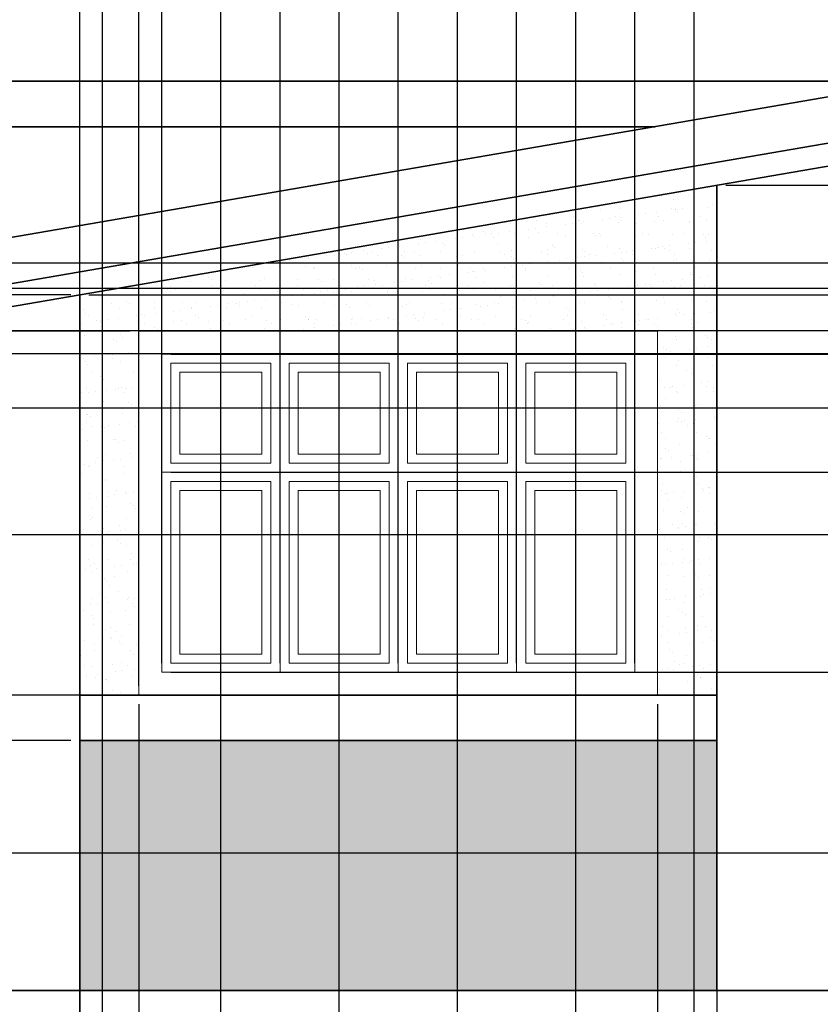
# Model space of a CAD drawing. Units: millimetres. Extents: x 937 to 4561, y 2711 to 5748.
# Tile 3 of 8: x 1663 to 2543, y 4062 to 5145. Entities that reach past the tile are written whole.
import ezdxf

# ---------------------------------------------------------------- set-up
doc = ezdxf.new("R2010")
doc.units = ezdxf.units.MM
doc.header["$MEASUREMENT"] = 0
for name, color, linetype, lineweight in [('A-ANNO-DIMS', 2, 'Continuous', 18), ('A-ELEV', 7, 'Continuous', 35), ('A-GLAZ', 4, 'Continuous', 18), ('A-ROOF', 1, 'Continuous', 35), ('A-WALL-PATT', 8, 'Continuous', 13)]:
    doc.layers.add(name, color=color, linetype=linetype, lineweight=lineweight)
doc.styles.get("Standard").update_dxf_attribs({"font": 'arial.ttf'})
doc.dimstyles.get("Standard").update_dxf_attribs({"dimtxt": 15, "dimasz": 10, "dimexe": 10, "dimexo": 10, "dimgap": 10, "dimtad": 0, "dimtih": 1, "dimtoh": 1, "dimdec": 0, "dimzin": 0, "dimdsep": 46, "dimtxsty": 'Standard', "dimcen": 5, "dimadec": 0, "dimazin": 0, "dimtfac": 1, "dimtdec": 0, "dimtofl": 0, "dimtmove": 0, "dimatfit": 3, "dimfxl": 1, "dimtolj": 1, "dimtzin": 0, "dimarcsym": 0})

# ---------------------------------------------------------------- blocks, each defined once
blk = doc.blocks.new('*D15')
at = {"layer": 'A-ANNO-DIMS', "color": 0, "lineweight": -2, "transparency": 16777216}
for p, q in [((1329.5, 4086.9), (1329.5, 5747.9)), ((4179.5, 5586.9), (4179.5, 5747.9)), ((1339.5, 5737.9), (2722, 5737.9)), ((4169.5, 5737.9), (2787, 5737.9))]:
    blk.add_line(p, q, dxfattribs=at)
at = {"layer": 'A-ANNO-DIMS', "color": 0, "transparency": 16777216}
for points in [[(1339.5, 5739.6), (1339.5, 5736.2), (1329.5, 5737.9)], [(4169.5, 5739.6), (4169.5, 5736.2), (4179.5, 5737.9)]]:
    blk.add_solid(points, dxfattribs=at)
at = {"layer": 'Defpoints', "color": 0, "transparency": 16777216}
for p in [(4179.5, 5737.9), (4179.5, 5576.9), (1329.5, 4076.9)]:
    blk.add_point(p, dxfattribs=at)
at = {"layer": 'A-ANNO-DIMS', "color": 0, "transparency": 16777216, "insert": (2754.5, 5737.9), "char_height": 15, "attachment_point": 5}
blk.add_mtext('\\A1;2850', dxfattribs=at)
blk = doc.blocks.new('*D16')
at = {"layer": 'A-ANNO-DIMS', "color": 0, "lineweight": -2, "transparency": 16777216}
for p, q in [((1329.5, 4859.2), (1329.5, 5747.9)), ((2947.4, 5137.7), (2947.4, 5747.9)), ((1339.5, 5737.9), (2106.8, 5737.9)), ((2937.4, 5737.9), (2170.2, 5737.9))]:
    blk.add_line(p, q, dxfattribs=at)
at = {"layer": 'A-ANNO-DIMS', "color": 0, "transparency": 16777216}
for points in [[(1339.5, 5739.6), (1339.5, 5736.2), (1329.5, 5737.9)], [(2937.4, 5739.6), (2937.4, 5736.2), (2947.4, 5737.9)]]:
    blk.add_solid(points, dxfattribs=at)
at = {"layer": 'Defpoints', "color": 0, "transparency": 16777216}
for p in [(2947.4, 5737.9), (2947.4, 5127.7), (1329.5, 4849.2)]:
    blk.add_point(p, dxfattribs=at)
at = {"layer": 'A-ANNO-DIMS', "color": 0, "transparency": 16777216, "insert": (2138.5, 5737.9), "char_height": 15, "attachment_point": 5}
blk.add_mtext('\\A1;1618', dxfattribs=at)
blk = doc.blocks.new('*D27')
at = {"layer": 'A-ANNO-DIMS', "color": 0, "lineweight": -2, "transparency": 16777216}
for p, q in [((1729.5, 4391.9), (1729.5, 2710.9)), ((1794.5, 4391.9), (1794.5, 2710.9)), ((1719.5, 2720.9), (1709.5, 2720.9)), ((1804.5, 2720.9), (1814.5, 2720.9))]:
    blk.add_line(p, q, dxfattribs=at)
at = {"layer": 'A-ANNO-DIMS', "color": 0, "transparency": 16777216}
for points in [[(1719.5, 2722.6), (1719.5, 2719.2), (1729.5, 2720.9)], [(1804.5, 2722.6), (1804.5, 2719.2), (1794.5, 2720.9)]]:
    blk.add_solid(points, dxfattribs=at)
at = {"layer": 'Defpoints', "color": 0, "transparency": 16777216}
for p in [(1729.5, 4401.9), (1794.5, 4401.9), (1794.5, 2720.9)]:
    blk.add_point(p, dxfattribs=at)
at = {"layer": 'A-ANNO-DIMS', "color": 0, "transparency": 16777216, "insert": (1762, 2720.9), "char_height": 15, "attachment_point": 5}
blk.add_mtext('\\A1;65', dxfattribs=at)
blk = doc.blocks.new('*D28')
at = {"layer": 'A-ANNO-DIMS', "color": 0, "lineweight": -2, "transparency": 16777216}
for p, q in [((1794.5, 4391.9), (1794.5, 2710.9)), ((2364.5, 4391.9), (2364.5, 2710.9)), ((1804.5, 2720.9), (2052.9, 2720.9)), ((2354.5, 2720.9), (2106, 2720.9))]:
    blk.add_line(p, q, dxfattribs=at)
at = {"layer": 'A-ANNO-DIMS', "color": 0, "transparency": 16777216}
for points in [[(1804.5, 2722.6), (1804.5, 2719.2), (1794.5, 2720.9)], [(2354.5, 2722.6), (2354.5, 2719.2), (2364.5, 2720.9)]]:
    blk.add_solid(points, dxfattribs=at)
at = {"layer": 'Defpoints', "color": 0, "transparency": 16777216}
for p in [(1794.5, 4401.9), (2364.5, 4401.9), (2364.5, 2720.9)]:
    blk.add_point(p, dxfattribs=at)
at = {"layer": 'A-ANNO-DIMS', "color": 0, "transparency": 16777216, "insert": (2079.5, 2720.9), "char_height": 15, "attachment_point": 5}
blk.add_mtext('\\A1;570', dxfattribs=at)
blk = doc.blocks.new('*D29')
at = {"layer": 'A-ANNO-DIMS', "color": 0, "lineweight": -2, "transparency": 16777216}
for p, q in [((2364.5, 4391.9), (2364.5, 2710.9)), ((2429.5, 4391.9), (2429.5, 2710.9)), ((2354.5, 2720.9), (2344.5, 2720.9)), ((2439.5, 2720.9), (2449.5, 2720.9))]:
    blk.add_line(p, q, dxfattribs=at)
at = {"layer": 'A-ANNO-DIMS', "color": 0, "transparency": 16777216}
for points in [[(2354.5, 2722.6), (2354.5, 2719.2), (2364.5, 2720.9)], [(2439.5, 2722.6), (2439.5, 2719.2), (2429.5, 2720.9)]]:
    blk.add_solid(points, dxfattribs=at)
at = {"layer": 'Defpoints', "color": 0, "transparency": 16777216}
for p in [(2364.5, 4401.9), (2429.5, 4401.9), (2429.5, 2720.9)]:
    blk.add_point(p, dxfattribs=at)
at = {"layer": 'A-ANNO-DIMS', "color": 0, "transparency": 16777216, "insert": (2397, 2720.9), "char_height": 15, "attachment_point": 5}
blk.add_mtext('\\A1;65', dxfattribs=at)
blk = doc.blocks.new('*D30')
at = {"layer": 'A-ANNO-DIMS', "color": 0, "lineweight": -2, "transparency": 16777216}
for p, q in [((1794.5, 4411.9), (1794.5, 5747.9)), ((1819.5, 4436.9), (1819.5, 5747.9)), ((1784.5, 5737.9), (1774.5, 5737.9)), ((1829.5, 5737.9), (1839.5, 5737.9))]:
    blk.add_line(p, q, dxfattribs=at)
at = {"layer": 'A-ANNO-DIMS', "color": 0, "transparency": 16777216}
for points in [[(1784.5, 5739.6), (1784.5, 5736.2), (1794.5, 5737.9)], [(1829.5, 5739.6), (1829.5, 5736.2), (1819.5, 5737.9)]]:
    blk.add_solid(points, dxfattribs=at)
at = {"layer": 'Defpoints', "color": 0, "transparency": 16777216}
for p in [(1819.5, 5737.9), (1819.5, 4426.9), (1794.5, 4401.9)]:
    blk.add_point(p, dxfattribs=at)
at = {"layer": 'A-ANNO-DIMS', "color": 0, "transparency": 16777216, "insert": (1860.4, 5737.9), "char_height": 15, "attachment_point": 5}
blk.add_mtext('\\A1;25', dxfattribs=at)
blk = doc.blocks.new('*D31')
at = {"layer": 'A-ANNO-DIMS', "color": 0, "lineweight": -2, "transparency": 16777216}
for p, q in [((1819.5, 4436.9), (1819.5, 5747.9)), ((1949.5, 4436.9), (1949.5, 5747.9)), ((1829.5, 5737.9), (1858.6, 5737.9)), ((1939.5, 5737.9), (1910.3, 5737.9))]:
    blk.add_line(p, q, dxfattribs=at)
at = {"layer": 'A-ANNO-DIMS', "color": 0, "transparency": 16777216}
for points in [[(1829.5, 5739.6), (1829.5, 5736.2), (1819.5, 5737.9)], [(1939.5, 5739.6), (1939.5, 5736.2), (1949.5, 5737.9)]]:
    blk.add_solid(points, dxfattribs=at)
at = {"layer": 'Defpoints', "color": 0, "transparency": 16777216}
for p in [(1949.5, 5737.9), (1819.5, 4426.9), (1949.5, 4426.9)]:
    blk.add_point(p, dxfattribs=at)
at = {"layer": 'A-ANNO-DIMS', "color": 0, "transparency": 16777216, "insert": (1884.5, 5737.9), "char_height": 15, "attachment_point": 5}
blk.add_mtext('\\A1;130', dxfattribs=at)
blk = doc.blocks.new('*D32')
at = {"layer": 'A-ANNO-DIMS', "color": 0, "lineweight": -2, "transparency": 16777216}
for p, q in [((1949.5, 4436.9), (1949.5, 5747.9)), ((2079.5, 4436.9), (2079.5, 5747.9)), ((1959.5, 5737.9), (1988.6, 5737.9)), ((2069.5, 5737.9), (2040.3, 5737.9))]:
    blk.add_line(p, q, dxfattribs=at)
at = {"layer": 'A-ANNO-DIMS', "color": 0, "transparency": 16777216}
for points in [[(1959.5, 5739.6), (1959.5, 5736.2), (1949.5, 5737.9)], [(2069.5, 5739.6), (2069.5, 5736.2), (2079.5, 5737.9)]]:
    blk.add_solid(points, dxfattribs=at)
at = {"layer": 'Defpoints', "color": 0, "transparency": 16777216}
for p in [(2079.5, 5737.9), (1949.5, 4426.9), (2079.5, 4426.9)]:
    blk.add_point(p, dxfattribs=at)
at = {"layer": 'A-ANNO-DIMS', "color": 0, "transparency": 16777216, "insert": (2014.5, 5737.9), "char_height": 15, "attachment_point": 5}
blk.add_mtext('\\A1;130', dxfattribs=at)
blk = doc.blocks.new('*D33')
at = {"layer": 'A-ANNO-DIMS', "color": 0, "lineweight": -2, "transparency": 16777216}
for p, q in [((2079.5, 4436.9), (2079.5, 5747.9)), ((2209.5, 4436.9), (2209.5, 5747.9)), ((2089.5, 5737.9), (2118.6, 5737.9)), ((2199.5, 5737.9), (2170.3, 5737.9))]:
    blk.add_line(p, q, dxfattribs=at)
at = {"layer": 'A-ANNO-DIMS', "color": 0, "transparency": 16777216}
for points in [[(2089.5, 5739.6), (2089.5, 5736.2), (2079.5, 5737.9)], [(2199.5, 5739.6), (2199.5, 5736.2), (2209.5, 5737.9)]]:
    blk.add_solid(points, dxfattribs=at)
at = {"layer": 'Defpoints', "color": 0, "transparency": 16777216}
for p in [(2209.5, 5737.9), (2079.5, 4426.9), (2209.5, 4426.9)]:
    blk.add_point(p, dxfattribs=at)
at = {"layer": 'A-ANNO-DIMS', "color": 0, "transparency": 16777216, "insert": (2144.5, 5737.9), "char_height": 15, "attachment_point": 5}
blk.add_mtext('\\A1;130', dxfattribs=at)
blk = doc.blocks.new('*D34')
at = {"layer": 'A-ANNO-DIMS', "color": 0, "lineweight": -2, "transparency": 16777216}
for p, q in [((2209.5, 4436.9), (2209.5, 5747.9)), ((2339.5, 4436.9), (2339.5, 5747.9)), ((2219.5, 5737.9), (2248.6, 5737.9)), ((2329.5, 5737.9), (2300.3, 5737.9))]:
    blk.add_line(p, q, dxfattribs=at)
at = {"layer": 'A-ANNO-DIMS', "color": 0, "transparency": 16777216}
for points in [[(2219.5, 5739.6), (2219.5, 5736.2), (2209.5, 5737.9)], [(2329.5, 5739.6), (2329.5, 5736.2), (2339.5, 5737.9)]]:
    blk.add_solid(points, dxfattribs=at)
at = {"layer": 'Defpoints', "color": 0, "transparency": 16777216}
for p in [(2339.5, 5737.9), (2209.5, 4426.9), (2339.5, 4426.9)]:
    blk.add_point(p, dxfattribs=at)
at = {"layer": 'A-ANNO-DIMS', "color": 0, "transparency": 16777216, "insert": (2274.5, 5737.9), "char_height": 15, "attachment_point": 5}
blk.add_mtext('\\A1;130', dxfattribs=at)
blk = doc.blocks.new('*D37')
at = {"layer": 'A-ANNO-DIMS', "color": 0, "lineweight": -2, "transparency": 16777216}
for p, q in [((1729.5, 3411.9), (1729.5, 5747.9)), ((1754.5, 3436.9), (1754.5, 5747.9)), ((1719.5, 5737.9), (1709.5, 5737.9)), ((1764.5, 5737.9), (1774.5, 5737.9))]:
    blk.add_line(p, q, dxfattribs=at)
at = {"layer": 'A-ANNO-DIMS', "color": 0, "transparency": 16777216}
for points in [[(1719.5, 5739.6), (1719.5, 5736.2), (1729.5, 5737.9)], [(1764.5, 5739.6), (1764.5, 5736.2), (1754.5, 5737.9)]]:
    blk.add_solid(points, dxfattribs=at)
at = {"layer": 'Defpoints', "color": 0, "transparency": 16777216}
for p in [(1754.5, 5737.9), (1754.5, 3426.9), (1729.5, 3401.9)]:
    blk.add_point(p, dxfattribs=at)
at = {"layer": 'A-ANNO-DIMS', "color": 0, "transparency": 16777216, "insert": (1795.4, 5737.9), "char_height": 15, "attachment_point": 5}
blk.add_mtext('\\A1;25', dxfattribs=at)
blk = doc.blocks.new('*D38')
at = {"layer": 'A-ANNO-DIMS', "color": 0, "lineweight": -2, "transparency": 16777216}
for p, q in [((1754.5, 3436.9), (1754.5, 5747.9)), ((1884.5, 3436.9), (1884.5, 5747.9)), ((1764.5, 5737.9), (1793.6, 5737.9)), ((1874.5, 5737.9), (1845.3, 5737.9))]:
    blk.add_line(p, q, dxfattribs=at)
at = {"layer": 'A-ANNO-DIMS', "color": 0, "transparency": 16777216}
for points in [[(1764.5, 5739.6), (1764.5, 5736.2), (1754.5, 5737.9)], [(1874.5, 5739.6), (1874.5, 5736.2), (1884.5, 5737.9)]]:
    blk.add_solid(points, dxfattribs=at)
at = {"layer": 'Defpoints', "color": 0, "transparency": 16777216}
for p in [(1884.5, 5737.9), (1754.5, 3426.9), (1884.5, 3426.9)]:
    blk.add_point(p, dxfattribs=at)
at = {"layer": 'A-ANNO-DIMS', "color": 0, "transparency": 16777216, "insert": (1819.5, 5737.9), "char_height": 15, "attachment_point": 5}
blk.add_mtext('\\A1;130', dxfattribs=at)
blk = doc.blocks.new('*D39')
at = {"layer": 'A-ANNO-DIMS', "color": 0, "lineweight": -2, "transparency": 16777216}
for p, q in [((1884.5, 3436.9), (1884.5, 5747.9)), ((2014.5, 3436.9), (2014.5, 5747.9)), ((1894.5, 5737.9), (1923.6, 5737.9)), ((2004.5, 5737.9), (1975.3, 5737.9))]:
    blk.add_line(p, q, dxfattribs=at)
at = {"layer": 'A-ANNO-DIMS', "color": 0, "transparency": 16777216}
for points in [[(1894.5, 5739.6), (1894.5, 5736.2), (1884.5, 5737.9)], [(2004.5, 5739.6), (2004.5, 5736.2), (2014.5, 5737.9)]]:
    blk.add_solid(points, dxfattribs=at)
at = {"layer": 'Defpoints', "color": 0, "transparency": 16777216}
for p in [(2014.5, 5737.9), (1884.5, 3426.9), (2014.5, 3426.9)]:
    blk.add_point(p, dxfattribs=at)
at = {"layer": 'A-ANNO-DIMS', "color": 0, "transparency": 16777216, "insert": (1949.5, 5737.9), "char_height": 15, "attachment_point": 5}
blk.add_mtext('\\A1;130', dxfattribs=at)
blk = doc.blocks.new('*D40')
at = {"layer": 'A-ANNO-DIMS', "color": 0, "lineweight": -2, "transparency": 16777216}
for p, q in [((2014.5, 3436.9), (2014.5, 5747.9)), ((2144.5, 3436.9), (2144.5, 5747.9)), ((2024.5, 5737.9), (2053.6, 5737.9)), ((2134.5, 5737.9), (2105.3, 5737.9))]:
    blk.add_line(p, q, dxfattribs=at)
at = {"layer": 'A-ANNO-DIMS', "color": 0, "transparency": 16777216}
for points in [[(2024.5, 5739.6), (2024.5, 5736.2), (2014.5, 5737.9)], [(2134.5, 5739.6), (2134.5, 5736.2), (2144.5, 5737.9)]]:
    blk.add_solid(points, dxfattribs=at)
at = {"layer": 'Defpoints', "color": 0, "transparency": 16777216}
for p in [(2144.5, 5737.9), (2014.5, 3426.9), (2144.5, 3426.9)]:
    blk.add_point(p, dxfattribs=at)
at = {"layer": 'A-ANNO-DIMS', "color": 0, "transparency": 16777216, "insert": (2079.5, 5737.9), "char_height": 15, "attachment_point": 5}
blk.add_mtext('\\A1;130', dxfattribs=at)
blk = doc.blocks.new('*D41')
at = {"layer": 'A-ANNO-DIMS', "color": 0, "lineweight": -2, "transparency": 16777216}
for p, q in [((2144.5, 3436.9), (2144.5, 5747.9)), ((2274.5, 3436.9), (2274.5, 5747.9)), ((2154.5, 5737.9), (2183.6, 5737.9)), ((2264.5, 5737.9), (2235.3, 5737.9))]:
    blk.add_line(p, q, dxfattribs=at)
at = {"layer": 'A-ANNO-DIMS', "color": 0, "transparency": 16777216}
for points in [[(2154.5, 5739.6), (2154.5, 5736.2), (2144.5, 5737.9)], [(2264.5, 5739.6), (2264.5, 5736.2), (2274.5, 5737.9)]]:
    blk.add_solid(points, dxfattribs=at)
at = {"layer": 'Defpoints', "color": 0, "transparency": 16777216}
for p in [(2274.5, 5737.9), (2144.5, 3426.9), (2274.5, 3426.9)]:
    blk.add_point(p, dxfattribs=at)
at = {"layer": 'A-ANNO-DIMS', "color": 0, "transparency": 16777216, "insert": (2209.5, 5737.9), "char_height": 15, "attachment_point": 5}
blk.add_mtext('\\A1;130', dxfattribs=at)
blk = doc.blocks.new('*D42')
at = {"layer": 'A-ANNO-DIMS', "color": 0, "lineweight": -2, "transparency": 16777216}
for p, q in [((2274.5, 3436.9), (2274.5, 5747.9)), ((2404.5, 3436.9), (2404.5, 5747.9)), ((2284.5, 5737.9), (2313.6, 5737.9)), ((2394.5, 5737.9), (2365.3, 5737.9))]:
    blk.add_line(p, q, dxfattribs=at)
at = {"layer": 'A-ANNO-DIMS', "color": 0, "transparency": 16777216}
for points in [[(2284.5, 5739.6), (2284.5, 5736.2), (2274.5, 5737.9)], [(2394.5, 5739.6), (2394.5, 5736.2), (2404.5, 5737.9)]]:
    blk.add_solid(points, dxfattribs=at)
at = {"layer": 'Defpoints', "color": 0, "transparency": 16777216}
for p in [(2404.5, 5737.9), (2274.5, 3426.9), (2404.5, 3426.9)]:
    blk.add_point(p, dxfattribs=at)
at = {"layer": 'A-ANNO-DIMS', "color": 0, "transparency": 16777216, "insert": (2339.5, 5737.9), "char_height": 15, "attachment_point": 5}
blk.add_mtext('\\A1;130', dxfattribs=at)
blk = doc.blocks.new('*D43')
at = {"layer": 'A-ANNO-DIMS', "color": 0, "lineweight": -2, "transparency": 16777216}
for p, q in [((1329.5, 4086.9), (1329.5, 5747.9)), ((2579.5, 4086.9), (2579.5, 5747.9)), ((1339.5, 5737.9), (1922.8, 5737.9)), ((2569.5, 5737.9), (1986.2, 5737.9))]:
    blk.add_line(p, q, dxfattribs=at)
at = {"layer": 'A-ANNO-DIMS', "color": 0, "transparency": 16777216}
for points in [[(1339.5, 5739.6), (1339.5, 5736.2), (1329.5, 5737.9)], [(2569.5, 5739.6), (2569.5, 5736.2), (2579.5, 5737.9)]]:
    blk.add_solid(points, dxfattribs=at)
at = {"layer": 'Defpoints', "color": 0, "transparency": 16777216}
for p in [(2579.5, 5737.9), (1329.5, 4076.9), (2579.5, 4076.9)]:
    blk.add_point(p, dxfattribs=at)
at = {"layer": 'A-ANNO-DIMS', "color": 0, "transparency": 16777216, "insert": (1954.5, 5737.9), "char_height": 15, "attachment_point": 5}
blk.add_mtext('\\A1;1250', dxfattribs=at)
blk = doc.blocks.new('*D60')
at = {"layer": 'A-ANNO-DIMS', "color": 0, "lineweight": -2, "transparency": 16777216}
for p, q in [((1784.5, 4401.9), (958.5, 4401.9)), ((968.5, 4391.9), (968.5, 4257.1)), ((968.5, 4086.9), (968.5, 4221.7)), ((1419.5, 4076.9), (958.5, 4076.9))]:
    blk.add_line(p, q, dxfattribs=at)
at = {"layer": 'A-ANNO-DIMS', "color": 0, "transparency": 16777216}
for points in [[(966.8, 4391.9), (970.2, 4391.9), (968.5, 4401.9)], [(966.8, 4086.9), (970.2, 4086.9), (968.5, 4076.9)]]:
    blk.add_solid(points, dxfattribs=at)
at = {"layer": 'Defpoints', "color": 0, "transparency": 16777216}
for p in [(968.5, 4401.9), (1794.5, 4401.9), (1429.5, 4076.9)]:
    blk.add_point(p, dxfattribs=at)
at = {"layer": 'A-ANNO-DIMS', "color": 0, "transparency": 16777216, "insert": (968.5, 4239.4), "char_height": 15, "attachment_point": 5}
blk.add_mtext('\\A1;325', dxfattribs=at)
blk = doc.blocks.new('*D61')
at = {"layer": 'A-ANNO-DIMS', "color": 0, "lineweight": -2, "transparency": 16777216}
for p, q in [((1784.5, 4801.9), (958.5, 4801.9)), ((968.5, 4791.9), (968.5, 4619.6)), ((968.5, 4411.9), (968.5, 4584.2)), ((1784.5, 4401.9), (958.5, 4401.9))]:
    blk.add_line(p, q, dxfattribs=at)
at = {"layer": 'A-ANNO-DIMS', "color": 0, "transparency": 16777216}
for points in [[(966.8, 4791.9), (970.2, 4791.9), (968.5, 4801.9)], [(966.8, 4411.9), (970.2, 4411.9), (968.5, 4401.9)]]:
    blk.add_solid(points, dxfattribs=at)
at = {"layer": 'Defpoints', "color": 0, "transparency": 16777216}
for p in [(968.5, 4801.9), (1794.5, 4801.9), (1794.5, 4401.9)]:
    blk.add_point(p, dxfattribs=at)
at = {"layer": 'A-ANNO-DIMS', "color": 0, "transparency": 16777216, "insert": (968.5, 4601.9), "char_height": 15, "attachment_point": 5}
blk.add_mtext('\\A1;400', dxfattribs=at)
blk = doc.blocks.new('*D62')
at = {"layer": 'A-ANNO-DIMS', "color": 0, "lineweight": -2, "transparency": 16777216}
for p, q in [((1419.5, 5076.9), (958.5, 5076.9)), ((968.5, 5066.9), (968.5, 4957.1)), ((968.5, 4811.9), (968.5, 4921.7)), ((1784.5, 4801.9), (958.5, 4801.9))]:
    blk.add_line(p, q, dxfattribs=at)
at = {"layer": 'A-ANNO-DIMS', "color": 0, "transparency": 16777216}
for points in [[(966.8, 5066.9), (970.2, 5066.9), (968.5, 5076.9)], [(966.8, 4811.9), (970.2, 4811.9), (968.5, 4801.9)]]:
    blk.add_solid(points, dxfattribs=at)
at = {"layer": 'Defpoints', "color": 0, "transparency": 16777216}
for p in [(968.5, 5076.9), (1429.5, 5076.9), (1794.5, 4801.9)]:
    blk.add_point(p, dxfattribs=at)
at = {"layer": 'A-ANNO-DIMS', "color": 0, "transparency": 16777216, "insert": (968.5, 4939.4), "char_height": 15, "attachment_point": 5}
blk.add_mtext('\\A1;275', dxfattribs=at)
blk = doc.blocks.new('*D63')
at = {"layer": 'A-ANNO-DIMS', "color": 0, "lineweight": -2, "transparency": 16777216}
for p, q in [((3169.5, 5576.9), (958.5, 5576.9)), ((968.5, 5566.9), (968.5, 5344.6)), ((968.5, 5086.9), (968.5, 5309.2)), ((1419.5, 5076.9), (958.5, 5076.9))]:
    blk.add_line(p, q, dxfattribs=at)
at = {"layer": 'A-ANNO-DIMS', "color": 0, "transparency": 16777216}
for points in [[(966.8, 5566.9), (970.2, 5566.9), (968.5, 5576.9)], [(966.8, 5086.9), (970.2, 5086.9), (968.5, 5076.9)]]:
    blk.add_solid(points, dxfattribs=at)
at = {"layer": 'Defpoints', "color": 0, "transparency": 16777216}
for p in [(968.5, 5576.9), (3179.5, 5576.9), (1429.5, 5076.9)]:
    blk.add_point(p, dxfattribs=at)
at = {"layer": 'A-ANNO-DIMS', "color": 0, "transparency": 16777216, "insert": (968.5, 5326.9), "char_height": 15, "attachment_point": 5}
blk.add_mtext('\\A1;500', dxfattribs=at)
blk = doc.blocks.new('*D68')
at = {"layer": 'A-ANNO-DIMS', "color": 0, "lineweight": -2, "transparency": 16777216}
for p, q in [((4490.5, 4812.8), (4490.5, 4822.8)), ((4490.5, 4822.8), (4500.5, 4822.8)), ((1364.5, 4802.8), (4500.5, 4802.8)), ((1364.5, 4777.4), (4500.5, 4777.4)), ((4490.5, 4767.4), (4490.5, 4757.4))]:
    blk.add_line(p, q, dxfattribs=at)
at = {"layer": 'A-ANNO-DIMS', "color": 0, "transparency": 16777216}
for points in [[(4488.8, 4812.8), (4492.2, 4812.8), (4490.5, 4802.8)], [(4488.8, 4767.4), (4492.2, 4767.4), (4490.5, 4777.4)]]:
    blk.add_solid(points, dxfattribs=at)
at = {"layer": 'Defpoints', "color": 0, "transparency": 16777216}
for p in [(1354.5, 4802.8), (4490.5, 4802.8), (1354.5, 4777.4)]:
    blk.add_point(p, dxfattribs=at)
at = {"layer": 'A-ANNO-DIMS', "color": 0, "transparency": 16777216, "insert": (4535.9, 4822.8), "char_height": 15, "attachment_point": 5}
blk.add_mtext('\\A1;25.37', dxfattribs=at)
blk = doc.blocks.new('*D69')
at = {"layer": 'A-ANNO-DIMS', "color": 0, "lineweight": -2, "transparency": 16777216}
for p, q in [((2957.4, 5127.7), (4500.5, 5127.7)), ((4490.5, 5117.7), (4490.5, 5006.1)), ((4490.5, 4859.2), (4490.5, 4970.8)), ((1339.5, 4849.2), (4500.5, 4849.2))]:
    blk.add_line(p, q, dxfattribs=at)
at = {"layer": 'A-ANNO-DIMS', "color": 0, "transparency": 16777216}
for points in [[(4488.8, 5117.7), (4492.2, 5117.7), (4490.5, 5127.7)], [(4488.8, 4859.2), (4492.2, 4859.2), (4490.5, 4849.2)]]:
    blk.add_solid(points, dxfattribs=at)
at = {"layer": 'Defpoints', "color": 0, "transparency": 16777216}
for p in [(2947.4, 5127.7), (4490.5, 5127.7), (1329.5, 4849.2)]:
    blk.add_point(p, dxfattribs=at)
at = {"layer": 'A-ANNO-DIMS', "color": 0, "transparency": 16777216, "insert": (4490.5, 4988.5), "char_height": 15, "attachment_point": 5}
blk.add_mtext('\\A1;278.45', dxfattribs=at)
blk = doc.blocks.new('*D74')
at = {"layer": 'A-ANNO-DIMS', "color": 0, "lineweight": -2, "transparency": 16777216}
for p, q in [((968.5, 4401.9), (968.5, 4411.9)), ((968.5, 4411.9), (978.5, 4411.9)), ((1719.5, 4401.9), (958.5, 4401.9)), ((968.5, 4361.9), (968.5, 4391.9)), ((1719.5, 4351.9), (958.5, 4351.9))]:
    blk.add_line(p, q, dxfattribs=at)
at = {"layer": 'A-ANNO-DIMS', "color": 0, "transparency": 16777216}
for points in [[(966.8, 4391.9), (970.2, 4391.9), (968.5, 4401.9)], [(966.8, 4361.9), (970.2, 4361.9), (968.5, 4351.9)]]:
    blk.add_solid(points, dxfattribs=at)
at = {"layer": 'Defpoints', "color": 0, "transparency": 16777216}
for p in [(968.5, 4401.9), (1729.5, 4401.9), (1729.5, 4351.9)]:
    blk.add_point(p, dxfattribs=at)
at = {"layer": 'A-ANNO-DIMS', "color": 0, "transparency": 16777216, "insert": (999.2, 4411.9), "char_height": 15, "attachment_point": 5}
blk.add_mtext('\\A1;50', dxfattribs=at)
blk = doc.blocks.new('*D75')
at = {"layer": 'A-ANNO-DIMS', "color": 0, "lineweight": -2, "transparency": 16777216}
for p, q in [((1829.5, 4646.9), (4500.5, 4646.9)), ((4490.5, 4636.9), (4490.5, 4554.6)), ((4490.5, 4436.9), (4490.5, 4519.2)), ((1829.5, 4426.9), (4500.5, 4426.9))]:
    blk.add_line(p, q, dxfattribs=at)
at = {"layer": 'A-ANNO-DIMS', "color": 0, "transparency": 16777216}
for points in [[(4488.8, 4636.9), (4492.2, 4636.9), (4490.5, 4646.9)], [(4488.8, 4436.9), (4492.2, 4436.9), (4490.5, 4426.9)]]:
    blk.add_solid(points, dxfattribs=at)
at = {"layer": 'Defpoints', "color": 0, "transparency": 16777216}
for p in [(1819.5, 4646.9), (4490.5, 4646.9), (1819.5, 4426.9)]:
    blk.add_point(p, dxfattribs=at)
at = {"layer": 'A-ANNO-DIMS', "color": 0, "transparency": 16777216, "insert": (4490.5, 4536.9), "char_height": 15, "attachment_point": 5}
blk.add_mtext('\\A1;220', dxfattribs=at)
blk = doc.blocks.new('*D76')
at = {"layer": 'A-ANNO-DIMS', "color": 0, "lineweight": -2, "transparency": 16777216}
for p, q in [((1829.5, 4776.9), (4500.5, 4776.9)), ((4490.5, 4766.9), (4490.5, 4729.6)), ((4490.5, 4656.9), (4490.5, 4694.2)), ((1829.5, 4646.9), (4500.5, 4646.9))]:
    blk.add_line(p, q, dxfattribs=at)
at = {"layer": 'A-ANNO-DIMS', "color": 0, "transparency": 16777216}
for points in [[(4488.8, 4766.9), (4492.2, 4766.9), (4490.5, 4776.9)], [(4488.8, 4656.9), (4492.2, 4656.9), (4490.5, 4646.9)]]:
    blk.add_solid(points, dxfattribs=at)
at = {"layer": 'Defpoints', "color": 0, "transparency": 16777216}
for p in [(1819.5, 4776.9), (4490.5, 4776.9), (1819.5, 4646.9)]:
    blk.add_point(p, dxfattribs=at)
at = {"layer": 'A-ANNO-DIMS', "color": 0, "transparency": 16777216, "insert": (4490.5, 4711.9), "char_height": 15, "attachment_point": 5}
blk.add_mtext('\\A1;130', dxfattribs=at)
blk = doc.blocks.new('*D77')
at = {"layer": 'A-ANNO-DIMS', "color": 0, "lineweight": -2, "transparency": 16777216}
for p, q in [((968.5, 4842), (968.5, 4852)), ((968.5, 4852), (978.5, 4852)), ((1719.5, 4842), (958.5, 4842)), ((968.5, 4811.9), (968.5, 4832)), ((1784.5, 4801.9), (958.5, 4801.9))]:
    blk.add_line(p, q, dxfattribs=at)
at = {"layer": 'A-ANNO-DIMS', "color": 0, "transparency": 16777216}
for points in [[(966.8, 4832), (970.2, 4832), (968.5, 4842)], [(966.8, 4811.9), (970.2, 4811.9), (968.5, 4801.9)]]:
    blk.add_solid(points, dxfattribs=at)
at = {"layer": 'Defpoints', "color": 0, "transparency": 16777216}
for p in [(968.5, 4842), (1729.5, 4842), (1794.5, 4801.9)]:
    blk.add_point(p, dxfattribs=at)
at = {"layer": 'A-ANNO-DIMS', "color": 0, "transparency": 16777216, "insert": (1014.1, 4852), "char_height": 15, "attachment_point": 5}
blk.add_mtext('\\A1;40.07', dxfattribs=at)
blk = doc.blocks.new('*D78')
at = {"layer": 'A-ANNO-DIMS', "color": 0, "lineweight": -2, "transparency": 16777216}
for p, q in [((2439.5, 4962.4), (4500.5, 4962.4)), ((4490.5, 4952.4), (4490.5, 4919.9)), ((4490.5, 4852), (4490.5, 4884.5)), ((1739.5, 4842), (4500.5, 4842))]:
    blk.add_line(p, q, dxfattribs=at)
at = {"layer": 'A-ANNO-DIMS', "color": 0, "transparency": 16777216}
for points in [[(4488.8, 4952.4), (4492.2, 4952.4), (4490.5, 4962.4)], [(4488.8, 4852), (4492.2, 4852), (4490.5, 4842)]]:
    blk.add_solid(points, dxfattribs=at)
at = {"layer": 'Defpoints', "color": 0, "transparency": 16777216}
for p in [(2429.5, 4962.4), (4490.5, 4962.4), (1729.5, 4842)]:
    blk.add_point(p, dxfattribs=at)
at = {"layer": 'A-ANNO-DIMS', "color": 0, "transparency": 16777216, "insert": (4490.5, 4902.2), "char_height": 15, "attachment_point": 5}
blk.add_mtext('\\A1;120.47', dxfattribs=at)
blk = doc.blocks.new('*D79')
at = {"layer": 'A-ANNO-DIMS', "color": 0, "lineweight": -2, "transparency": 16777216}
for p, q in [((3019.5, 4876.9), (958.5, 4876.9)), ((968.5, 4866.9), (968.5, 4814.8)), ((968.5, 4727.5), (968.5, 4779.5)), ((2569.5, 4717.5), (958.5, 4717.5))]:
    blk.add_line(p, q, dxfattribs=at)
at = {"layer": 'A-ANNO-DIMS', "color": 0, "transparency": 16777216}
for points in [[(966.8, 4866.9), (970.2, 4866.9), (968.5, 4876.9)], [(966.8, 4727.5), (970.2, 4727.5), (968.5, 4717.5)]]:
    blk.add_solid(points, dxfattribs=at)
at = {"layer": 'Defpoints', "color": 0, "transparency": 16777216}
for p in [(968.5, 4876.9), (3029.5, 4876.9), (2579.5, 4717.5)]:
    blk.add_point(p, dxfattribs=at)
at = {"layer": 'A-ANNO-DIMS', "color": 0, "transparency": 16777216, "insert": (968.5, 4797.2), "char_height": 15, "attachment_point": 5}
blk.add_mtext('\\A1;159.44', dxfattribs=at)
blk = doc.blocks.new('*D86')
at = {"layer": 'A-ANNO-DIMS', "color": 0, "lineweight": -2, "transparency": 16777216}
for p, q in [((968.5, 4076.9), (968.5, 4086.9)), ((968.5, 4086.9), (978.5, 4086.9)), ((2569.5, 4076.9), (958.5, 4076.9)), ((968.5, 4036.9), (968.5, 4066.9)), ((2569.5, 4026.9), (958.5, 4026.9))]:
    blk.add_line(p, q, dxfattribs=at)
at = {"layer": 'A-ANNO-DIMS', "color": 0, "transparency": 16777216}
for points in [[(966.8, 4066.9), (970.2, 4066.9), (968.5, 4076.9)], [(966.8, 4036.9), (970.2, 4036.9), (968.5, 4026.9)]]:
    blk.add_solid(points, dxfattribs=at)
at = {"layer": 'Defpoints', "color": 0, "transparency": 16777216}
for p in [(968.5, 4076.9), (2579.5, 4076.9), (2579.5, 4026.9)]:
    blk.add_point(p, dxfattribs=at)
at = {"layer": 'A-ANNO-DIMS', "color": 0, "transparency": 16777216, "insert": (999.2, 4086.9), "char_height": 15, "attachment_point": 5}
blk.add_mtext('\\A1;50', dxfattribs=at)
blk = doc.blocks.new('*D87')
at = {"layer": 'A-ANNO-DIMS', "color": 0, "lineweight": -2, "transparency": 16777216}
for p, q in [((2794.5, 4227.9), (958.5, 4227.9)), ((968.5, 4217.9), (968.5, 4170.1)), ((968.5, 4086.9), (968.5, 4134.7)), ((2719.5, 4076.9), (958.5, 4076.9))]:
    blk.add_line(p, q, dxfattribs=at)
at = {"layer": 'A-ANNO-DIMS', "color": 0, "transparency": 16777216}
for points in [[(966.8, 4217.9), (970.2, 4217.9), (968.5, 4227.9)], [(966.8, 4086.9), (970.2, 4086.9), (968.5, 4076.9)]]:
    blk.add_solid(points, dxfattribs=at)
at = {"layer": 'Defpoints', "color": 0, "transparency": 16777216}
for p in [(968.5, 4227.9), (2804.5, 4227.9), (2729.5, 4076.9)]:
    blk.add_point(p, dxfattribs=at)
at = {"layer": 'A-ANNO-DIMS', "color": 0, "transparency": 16777216, "insert": (968.5, 4152.4), "char_height": 15, "attachment_point": 5}
blk.add_mtext('\\A1;151', dxfattribs=at)
blk = doc.blocks.new('*D93')
at = {"layer": 'A-ANNO-DIMS', "color": 0, "lineweight": -2, "transparency": 16777216}
for p, q in [((2794.5, 4577.9), (958.5, 4577.9)), ((968.5, 4567.9), (968.5, 4420.6)), ((968.5, 4237.9), (968.5, 4385.2)), ((2794.5, 4227.9), (958.5, 4227.9))]:
    blk.add_line(p, q, dxfattribs=at)
at = {"layer": 'A-ANNO-DIMS', "color": 0, "transparency": 16777216}
for points in [[(966.8, 4567.9), (970.2, 4567.9), (968.5, 4577.9)], [(966.8, 4237.9), (970.2, 4237.9), (968.5, 4227.9)]]:
    blk.add_solid(points, dxfattribs=at)
at = {"layer": 'Defpoints', "color": 0, "transparency": 16777216}
for p in [(968.5, 4577.9), (2804.5, 4577.9), (2804.5, 4227.9)]:
    blk.add_point(p, dxfattribs=at)
at = {"layer": 'A-ANNO-DIMS', "color": 0, "transparency": 16777216, "insert": (968.5, 4402.9), "char_height": 15, "attachment_point": 5}
blk.add_mtext('\\A1;350', dxfattribs=at)

msp = doc.modelspace()

# ---------------------------------------------------------------- hatches: boundary and pattern name
at = {"layer": 'A-WALL-PATT'}
h = msp.add_hatch(dxfattribs=at)
h.set_pattern_fill('AR-SAND', color=256, scale=15)
h.paths.add_polyline_path([(2429.4852, 4962.4414), (1729.4852, 4841.9734), (1729.4852, 4401.9013), (1794.4852, 4401.9013), (1794.4852, 4801.9013), (2079.4852, 4801.9013), (2364.4852, 4801.9013), (2364.4852, 4401.9013), (2429.4852, 4401.9013)])
h = msp.add_hatch(dxfattribs=at)
h.set_pattern_fill('AR-SAND', color=256, scale=15)
h.paths.add_polyline_path([(2429.4852, 4351.9013), (2364.4852, 4351.9013), (1729.4852, 4351.9013), (1729.4852, 4076.9013), (2429.4852, 4076.9013)])
h.paths.add_polyline_path([(2479.4852, 3926.9013), (1679.4852, 3926.9013), (1679.4852, 3401.9013), (1729.4852, 3401.9013), (1729.4852, 3801.9013), (2429.4852, 3801.9013), (2429.4852, 3401.9013), (2479.4852, 3401.9013)])
h.paths.add_polyline_path([(2479.4852, 3351.9013), (1679.4852, 3351.9013), (1679.4852, 3076.9013), (2479.4852, 3076.9013)])

# ---------------------------------------------------------------- linework, layer by layer
at = {"layer": 'A-ELEV'}
for p, q in [((2429.4852, 4076.9013), (2429.4852, 4962.4414)), ((1729.4852, 4076.9013), (1729.4852, 4841.9734)), ((1729.4852, 4401.9013), (2429.4852, 4401.9013)), ((1729.4852, 4351.9013), (2429.4852, 4351.9013)), ((2429.4852, 4351.9013), (2364.4852, 4351.9013)), ((1429.4852, 4076.9013), (3479.4852, 4076.9013)), ((2729.4852, 4076.9013), (2479.4852, 4076.9013))]:
    msp.add_line(p, q, dxfattribs=at)
at = {"layer": 'A-GLAZ'}
for p, q in [((1794.4852, 4801.9013), (2079.4852, 4801.9013)), ((1794.4852, 4401.9013), (1794.4852, 4801.9013)), ((2079.4852, 4801.9013), (2364.4852, 4801.9013)), ((2364.4852, 4801.9013), (2364.4852, 4401.9013)), ((1819.4852, 4776.9013), (2079.4852, 4776.9013)), ((1819.4852, 4426.9013), (1819.4852, 4776.9013)), ((1819.4852, 4776.9013), (1949.4852, 4776.9013)), ((1819.4852, 4646.9013), (1819.4852, 4776.9013)), ((1949.4852, 4776.9013), (1949.4852, 4426.9013)), ((1949.4852, 4776.9013), (1949.4852, 4646.9013)), ((1949.4852, 4776.9013), (2079.4852, 4776.9013)), ((1949.4852, 4646.9013), (1949.4852, 4776.9013)), ((2079.4852, 4776.9013), (2079.4852, 4426.9013)), ((2079.4852, 4776.9013), (2079.4852, 4426.9013)), ((2079.4852, 4776.9013), (2079.4852, 4646.9013)), ((2079.4852, 4776.9013), (2209.4852, 4776.9013)), ((2079.4852, 4646.9013), (2079.4852, 4776.9013)), ((2079.4852, 4776.9013), (2339.4852, 4776.9013)), ((2209.4852, 4776.9013), (2209.4852, 4426.9013)), ((2209.4852, 4776.9013), (2209.4852, 4646.9013)), ((2209.4852, 4776.9013), (2339.4852, 4776.9013)), ((2209.4852, 4646.9013), (2209.4852, 4776.9013)), ((2339.4852, 4776.9013), (2339.4852, 4426.9013)), ((2339.4852, 4776.9013), (2339.4852, 4646.9013)), ((1829.4852, 4766.9013), (1939.4852, 4766.9013)), ((1829.4852, 4656.9013), (1829.4852, 4766.9013)), ((1939.4852, 4766.9013), (1939.4852, 4656.9013)), ((1959.4852, 4766.9013), (2069.4852, 4766.9013)), ((1959.4852, 4656.9013), (1959.4852, 4766.9013)), ((2069.4852, 4766.9013), (2069.4852, 4656.9013)), ((2089.4852, 4766.9013), (2199.4852, 4766.9013)), ((2089.4852, 4656.9013), (2089.4852, 4766.9013)), ((2199.4852, 4766.9013), (2199.4852, 4656.9013)), ((2219.4852, 4766.9013), (2329.4852, 4766.9013)), ((2219.4852, 4656.9013), (2219.4852, 4766.9013)), ((2329.4852, 4766.9013), (2329.4852, 4656.9013)), ((1839.4852, 4756.9013), (1929.4852, 4756.9013)), ((1839.4852, 4666.9013), (1839.4852, 4756.9013)), ((1929.4852, 4756.9013), (1929.4852, 4666.9013)), ((1969.4852, 4756.9013), (2059.4852, 4756.9013)), ((1969.4852, 4666.9013), (1969.4852, 4756.9013)), ((2059.4852, 4756.9013), (2059.4852, 4666.9013)), ((2099.4852, 4756.9013), (2189.4852, 4756.9013)), ((2099.4852, 4666.9013), (2099.4852, 4756.9013)), ((2189.4852, 4756.9013), (2189.4852, 4666.9013)), ((2229.4852, 4756.9013), (2319.4852, 4756.9013)), ((2229.4852, 4666.9013), (2229.4852, 4756.9013)), ((2319.4852, 4756.9013), (2319.4852, 4666.9013)), ((1929.4852, 4666.9013), (1839.4852, 4666.9013)), ((2059.4852, 4666.9013), (1969.4852, 4666.9013)), ((2189.4852, 4666.9013), (2099.4852, 4666.9013)), ((2319.4852, 4666.9013), (2229.4852, 4666.9013)), ((1939.4852, 4656.9013), (1829.4852, 4656.9013)), ((2069.4852, 4656.9013), (1959.4852, 4656.9013)), ((2199.4852, 4656.9013), (2089.4852, 4656.9013)), ((2329.4852, 4656.9013), (2219.4852, 4656.9013)), ((1819.4852, 4646.9013), (2079.4852, 4646.9013)), ((1949.4852, 4646.9013), (1819.4852, 4646.9013)), ((1819.4852, 4646.9013), (1949.4852, 4646.9013)), ((1819.4852, 4426.9013), (1819.4852, 4646.9013)), ((2079.4852, 4646.9013), (1949.4852, 4646.9013)), ((1949.4852, 4646.9013), (1949.4852, 4426.9013)), ((1949.4852, 4646.9013), (2079.4852, 4646.9013)), ((1949.4852, 4426.9013), (1949.4852, 4646.9013)), ((2209.4852, 4646.9013), (2079.4852, 4646.9013)), ((2079.4852, 4646.9013), (2079.4852, 4426.9013)), ((2079.4852, 4646.9013), (2209.4852, 4646.9013)), ((2079.4852, 4426.9013), (2079.4852, 4646.9013)), ((2079.4852, 4646.9013), (2339.4852, 4646.9013)), ((2339.4852, 4646.9013), (2209.4852, 4646.9013)), ((2209.4852, 4646.9013), (2209.4852, 4426.9013)), ((2209.4852, 4646.9013), (2339.4852, 4646.9013)), ((2209.4852, 4426.9013), (2209.4852, 4646.9013)), ((2339.4852, 4646.9013), (2339.4852, 4426.9013)), ((1829.4852, 4636.9013), (1939.4852, 4636.9013)), ((1829.4852, 4436.9013), (1829.4852, 4636.9013)), ((1939.4852, 4636.9013), (1939.4852, 4436.9013)), ((1959.4852, 4636.9013), (2069.4852, 4636.9013)), ((1959.4852, 4436.9013), (1959.4852, 4636.9013)), ((2069.4852, 4636.9013), (2069.4852, 4436.9013)), ((2089.4852, 4636.9013), (2199.4852, 4636.9013)), ((2089.4852, 4436.9013), (2089.4852, 4636.9013)), ((2199.4852, 4636.9013), (2199.4852, 4436.9013)), ((2219.4852, 4636.9013), (2329.4852, 4636.9013)), ((2219.4852, 4436.9013), (2219.4852, 4636.9013)), ((2329.4852, 4636.9013), (2329.4852, 4436.9013)), ((1839.4852, 4626.9013), (1929.4852, 4626.9013)), ((1839.4852, 4446.9013), (1839.4852, 4626.9013)), ((1929.4852, 4626.9013), (1929.4852, 4446.9013)), ((1969.4852, 4626.9013), (2059.4852, 4626.9013)), ((1969.4852, 4446.9013), (1969.4852, 4626.9013)), ((2059.4852, 4626.9013), (2059.4852, 4446.9013)), ((2099.4852, 4626.9013), (2189.4852, 4626.9013)), ((2099.4852, 4446.9013), (2099.4852, 4626.9013)), ((2189.4852, 4626.9013), (2189.4852, 4446.9013)), ((2229.4852, 4626.9013), (2319.4852, 4626.9013)), ((2229.4852, 4446.9013), (2229.4852, 4626.9013)), ((2319.4852, 4626.9013), (2319.4852, 4446.9013)), ((1929.4852, 4446.9013), (1839.4852, 4446.9013)), ((2059.4852, 4446.9013), (1969.4852, 4446.9013)), ((2189.4852, 4446.9013), (2099.4852, 4446.9013)), ((2319.4852, 4446.9013), (2229.4852, 4446.9013)), ((1939.4852, 4436.9013), (1829.4852, 4436.9013)), ((2069.4852, 4436.9013), (1959.4852, 4436.9013)), ((2199.4852, 4436.9013), (2089.4852, 4436.9013)), ((2329.4852, 4436.9013), (2219.4852, 4436.9013)), ((1949.4852, 4426.9013), (1819.4852, 4426.9013)), ((2079.4852, 4426.9013), (1819.4852, 4426.9013)), ((2079.4852, 4426.9013), (1949.4852, 4426.9013)), ((2339.4852, 4426.9013), (2079.4852, 4426.9013)), ((2209.4852, 4426.9013), (2079.4852, 4426.9013)), ((2339.4852, 4426.9013), (2209.4852, 4426.9013)), ((2079.4852, 4401.9013), (1794.4852, 4401.9013)), ((2364.4852, 4401.9013), (2079.4852, 4401.9013))]:
    msp.add_line(p, q, dxfattribs=at)
at = {"layer": 'A-ROOF'}
for p, q in [((2947.4456, 5127.6834), (1329.4852, 4849.2371)), ((2947.1723, 5076.9013), (1329.4852, 4798.5021)), ((1429.4852, 5076.9013), (2652.3676, 5076.9013)), ((2922.0122, 5047.2038), (1354.4852, 4777.437)), ((1429.4852, 5026.9013), (2361.834, 5026.9013))]:
    msp.add_line(p, q, dxfattribs=at)

# ---------------------------------------------------------------- dimensions: what is measured, and where the dimension line sits
at = {"layer": 'A-ANNO-DIMS'}
for base, p1, p2, picture, middle in [((4179.4852, 5737.9013), (1329.4852, 4076.9013), (4179.4852, 5576.9013), '*D15', (2754.4852, 5737.9013)), ((2947.4456, 5737.9013), (1329.4852, 4849.2371), (2947.4456, 5127.6834), '*D16', (2138.4654, 5737.9013)), ((2579.4852, 5737.9013), (1329.4852, 4076.9013), (2579.4852, 4076.9013), '*D43', (1954.4852, 5737.9013)), ((1754.4852, 5737.9013), (1729.4852, 3401.9013), (1754.4852, 3426.9013), '*D37', (1795.4129, 5737.9013)), ((1884.4852, 5737.9013), (1754.4852, 3426.9013), (1884.4852, 3426.9013), '*D38', (1819.4852, 5737.9013)), ((1819.4852, 5737.9013), (1794.4852, 4401.9013), (1819.4852, 4426.9013), '*D30', (1860.4129, 5737.9013)), ((1949.4852, 5737.9013), (1819.4852, 4426.9013), (1949.4852, 4426.9013), '*D31', (1884.4852, 5737.9013)), ((2014.4852, 5737.9013), (1884.4852, 3426.9013), (2014.4852, 3426.9013), '*D39', (1949.4852, 5737.9013)), ((2079.4852, 5737.9013), (1949.4852, 4426.9013), (2079.4852, 4426.9013), '*D32', (2014.4852, 5737.9013)), ((2144.4852, 5737.9013), (2014.4852, 3426.9013), (2144.4852, 3426.9013), '*D40', (2079.4852, 5737.9013)), ((2209.4852, 5737.9013), (2079.4852, 4426.9013), (2209.4852, 4426.9013), '*D33', (2144.4852, 5737.9013)), ((2274.4852, 5737.9013), (2144.4852, 3426.9013), (2274.4852, 3426.9013), '*D41', (2209.4852, 5737.9013)), ((2339.4852, 5737.9013), (2209.4852, 4426.9013), (2339.4852, 4426.9013), '*D34', (2274.4852, 5737.9013)), ((2404.4852, 5737.9013), (2274.4852, 3426.9013), (2404.4852, 3426.9013), '*D42', (2339.4852, 5737.9013)), ((1794.4852, 2720.9013), (1729.4852, 4401.9013), (1794.4852, 4401.9013), '*D27', (1761.9852, 2720.9013)), ((2364.4852, 2720.9013), (1794.4852, 4401.9013), (2364.4852, 4401.9013), '*D28', (2079.4852, 2720.9013)), ((2429.4852, 2720.9013), (2364.4852, 4401.9013), (2429.4852, 4401.9013), '*D29', (2396.9852, 2720.9013))]:
    dim = msp.add_linear_dim(base=base, p1=p1, p2=p2, dimstyle='Standard', override={"dimdec": 0, "dimlfac": 1, "dimrnd": 0, "dimzin": 0, "dimdsep": 46, "dimlunit": 2}, dxfattribs=at)
    dim.commit()
    dim.dimension.update_dxf_attribs({"geometry": picture, "text_midpoint": middle})
for base, p1, p2, override, picture, middle in [((968.4852, 5576.9013), (1429.4852, 5076.9013), (3179.4852, 5576.9013), {"dimdec": 0, "dimlfac": 1, "dimrnd": 0, "dimzin": 0, "dimdsep": 46, "dimlunit": 2}, '*D63', (968.4852, 5326.9013)), ((4490.4852, 5127.6834), (1329.4852, 4849.2371), (2947.4456, 5127.6834), {"dimdec": 2, "dimlfac": 1, "dimrnd": 0, "dimzin": 0, "dimdsep": 46, "dimlunit": 2}, '*D69', (4490.4852, 4988.4602)), ((968.4852, 5076.9013), (1794.4852, 4801.9013), (1429.4852, 5076.9013), {"dimdec": 0, "dimlfac": 1, "dimrnd": 0, "dimzin": 0, "dimdsep": 46, "dimlunit": 2}, '*D62', (968.4852, 4939.4013)), ((4490.4852, 4962.4414), (1729.4852, 4841.9734), (2429.4852, 4962.4414), {"dimdec": 2, "dimlfac": 1, "dimrnd": 0, "dimzin": 0, "dimdsep": 46, "dimlunit": 2}, '*D78', (4490.4852, 4902.2074)), ((968.4852, 4876.9013), (2579.4852, 4717.4604), (3029.4852, 4876.9013), {"dimdec": 2, "dimlfac": 1, "dimrnd": 0, "dimzin": 0, "dimdsep": 46, "dimlunit": 2}, '*D79', (968.4852, 4797.1808)), ((968.4852, 4841.9734), (1794.4852, 4801.9013), (1729.4852, 4841.9734), {"dimdec": 2, "dimlfac": 1, "dimrnd": 0, "dimzin": 0, "dimdsep": 46, "dimlunit": 2}, '*D77', (1014.0957, 4851.9734)), ((4490.4852, 4802.8045), (1354.4852, 4777.437), (1354.4852, 4802.8045), {"dimdec": 2, "dimlfac": 1, "dimrnd": 0, "dimzin": 0, "dimdsep": 46, "dimlunit": 2}, '*D68', (4535.9218, 4822.8045)), ((968.4852, 4801.9013), (1794.4852, 4401.9013), (1794.4852, 4801.9013), {"dimdec": 0, "dimlfac": 1, "dimrnd": 0, "dimzin": 0, "dimdsep": 46, "dimlunit": 2}, '*D61', (968.4852, 4601.9013)), ((4490.4852, 4776.9013), (1819.4852, 4646.9013), (1819.4852, 4776.9013), {"dimdec": 0, "dimlfac": 1, "dimrnd": 0, "dimzin": 0, "dimdsep": 46, "dimlunit": 2}, '*D76', (4490.4852, 4711.9013)), ((4490.4852, 4646.9013), (1819.4852, 4426.9013), (1819.4852, 4646.9013), {"dimdec": 0, "dimlfac": 1, "dimrnd": 0, "dimzin": 0, "dimdsep": 46, "dimlunit": 2}, '*D75', (4490.4852, 4536.9013)), ((968.4852, 4577.9047), (2804.4852, 4227.9047), (2804.4852, 4577.9047), {"dimdec": 0, "dimlfac": 1, "dimrnd": 0, "dimzin": 0, "dimdsep": 46, "dimlunit": 2}, '*D93', (968.4852, 4402.9047)), ((968.4852, 4401.9013), (1729.4852, 4351.9013), (1729.4852, 4401.9013), {"dimdec": 0, "dimlfac": 1, "dimrnd": 0, "dimzin": 0, "dimdsep": 46, "dimlunit": 2}, '*D74', (999.2031, 4411.9013)), ((968.4852, 4401.9013), (1429.4852, 4076.9013), (1794.4852, 4401.9013), {"dimdec": 0, "dimlfac": 1, "dimrnd": 0, "dimzin": 0, "dimdsep": 46, "dimlunit": 2}, '*D60', (968.4852, 4239.4013)), ((968.4852, 4227.9047), (2729.4852, 4076.9013), (2804.4852, 4227.9047), {"dimdec": 0, "dimlfac": 1, "dimrnd": 0, "dimzin": 0, "dimdsep": 46, "dimlunit": 2}, '*D87', (968.4852, 4152.403)), ((968.4852, 4076.9013), (2579.4852, 4026.9013), (2579.4852, 4076.9013), {"dimdec": 0, "dimlfac": 1, "dimrnd": 0, "dimzin": 0, "dimdsep": 46, "dimlunit": 2}, '*D86', (999.2031, 4086.9013))]:
    dim = msp.add_linear_dim(base=base, p1=p1, p2=p2, angle=90, dimstyle='Standard', override=override, dxfattribs=at)
    dim.commit()
    dim.dimension.update_dxf_attribs({"geometry": picture, "text_midpoint": middle})

doc.saveas('drawing.dxf')
